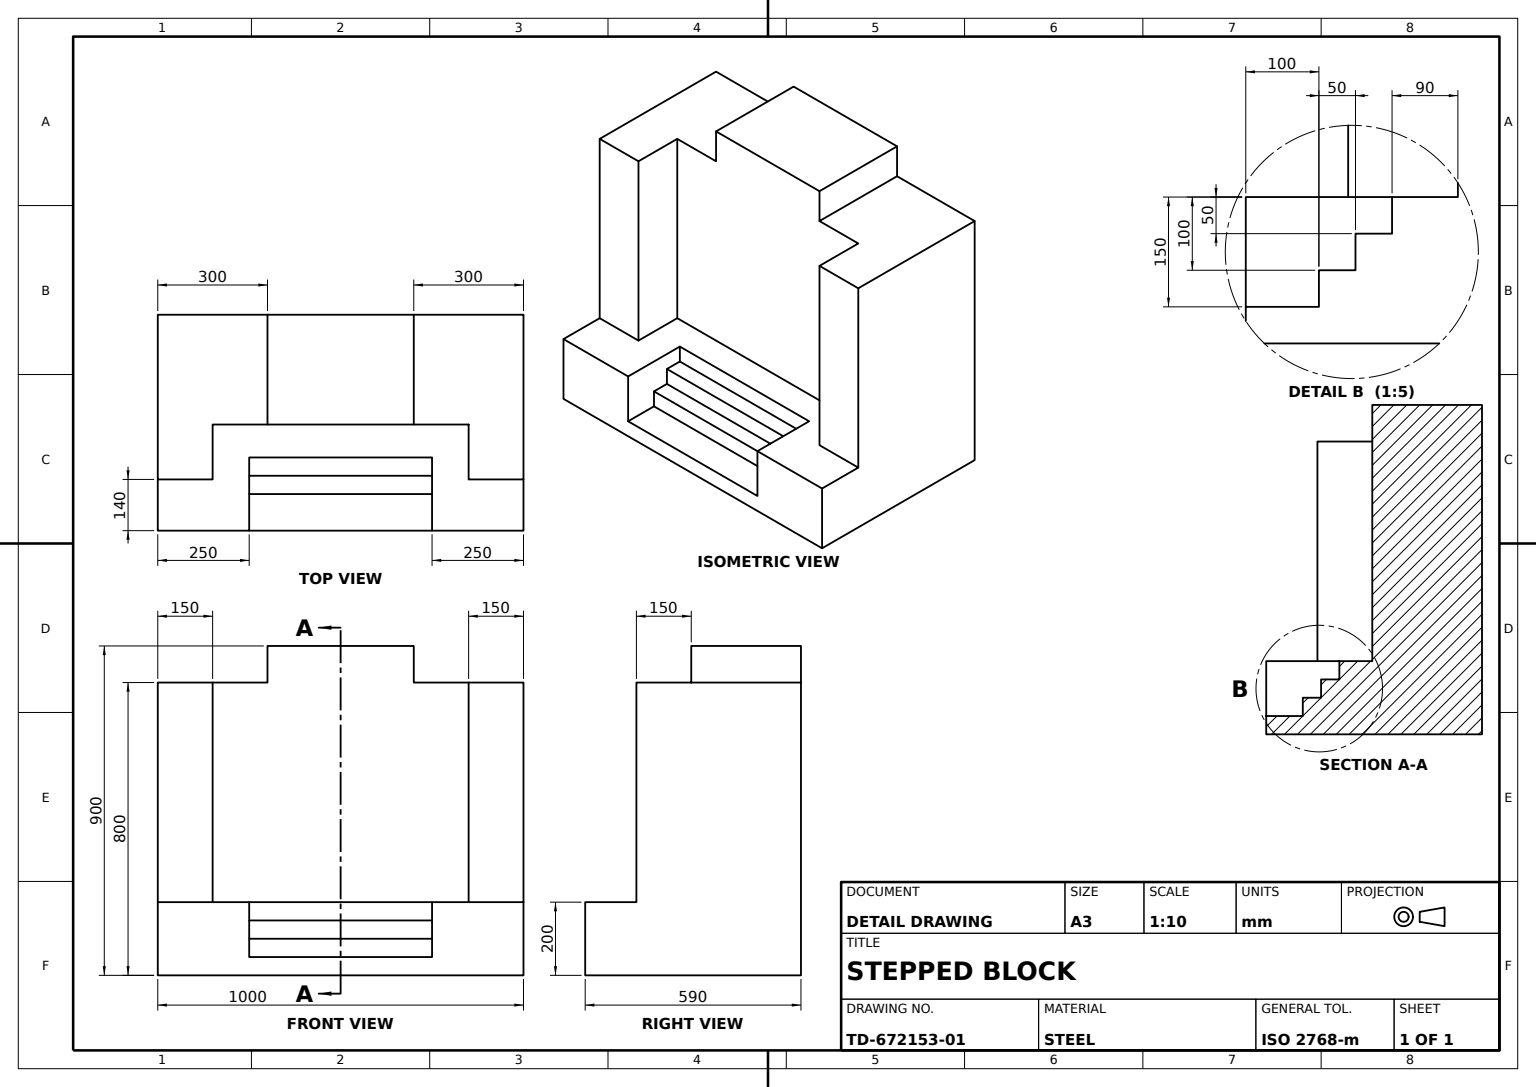
from build123d import *

# Parameters (mm, degrees)
BASE_BLOCK_DEPTH          = 1000
SIDE_BOSS_A_SKETCH_W      = 150
SIDE_BOSS_A_SKETCH_H      = 600
SIDE_BOSS_A_DEPTH         = 150
SIDE_BOSS_B_SKETCH_W      = 150
SIDE_BOSS_B_SKETCH_H      = 600
SIDE_BOSS_B_DEPTH         = 150
CORNER_BOSS_DEPTH         = 100
TOP_STEP_CUT_DEPTH        = 150
TOP_GROOVE_CUT_DEPTH      = 1450.689621954
TOP_GROOVE_CUT_DEPTH_BACK = 100
GROOVE_NOTCH_SKETCH_W     = 500
GROOVE_NOTCH_SKETCH_H     = 50
GROOVE_NOTCH_CUT_DEPTH    = 50
GROOVE_INFILL_BOSS_DEPTH  = 50


with BuildPart() as part:
    # Base Profile Sketch → Base Block (new body)
    with BuildSketch(Plane.XY):
        Polygon((0, 0), (540, 0), (540, 800), (240, 800), (240, 200), (0, 200), align=None)
    extrude(amount=BASE_BLOCK_DEPTH)

    # Side Boss A Sketch → Side Boss A (add)
    with BuildSketch(Plane(origin=(0, 0, 0), x_dir=(-1, 0, 0), z_dir=(0, 0, -1))):
        with Locations((-165, 500)):
            Rectangle(SIDE_BOSS_A_SKETCH_W, SIDE_BOSS_A_SKETCH_H)
    extrude(amount=-SIDE_BOSS_A_DEPTH)

    # Side Boss B Sketch → Side Boss B (add)
    with BuildSketch(Plane.XY.offset(1000)):
        with Locations((165, 500)):
            Rectangle(SIDE_BOSS_B_SKETCH_W, SIDE_BOSS_B_SKETCH_H)
    extrude(amount=-SIDE_BOSS_B_DEPTH)

    # Corner Boss Sketch → Corner Boss (add)
    with BuildSketch(Plane(origin=(0, 800, 0), x_dir=(1, 0, 0), z_dir=(0, 1, 0))):
        Polygon((540, -500), (540, -300), (240, -300), (240, -700), (540, -700), align=None)
    extrude(amount=CORNER_BOSS_DEPTH)

    # Top Step Cut Sketch → Top Step Cut (cut)
    with BuildSketch(Plane.ZY):
        Polygon((500, 200), (250, 200), (250, 150), (750, 150), (750, 200), align=None)
    extrude(amount=-TOP_STEP_CUT_DEPTH, mode=Mode.SUBTRACT)

    # Top Groove Sketch → Top Groove Cut (cut, two sides: drawn at the far end of the back side and taken through both)
    with BuildSketch(Plane.ZY.offset(-TOP_GROOVE_CUT_DEPTH_BACK)):
        Polygon((250, 2281.32034356), (250, 150), (250, 100), (750, 100), (750, 150), (750, 2281.32034356), (750, 6543.961030679), (250, 6543.961030679), align=None)
    extrude(amount=TOP_GROOVE_CUT_DEPTH + TOP_GROOVE_CUT_DEPTH_BACK, mode=Mode.SUBTRACT)

    # Groove Notch Sketch → Groove Notch Cut (cut)
    with BuildSketch(Plane.ZY):
        with Locations((500, 75)):
            Rectangle(GROOVE_NOTCH_SKETCH_W, GROOVE_NOTCH_SKETCH_H)
    extrude(amount=-GROOVE_NOTCH_CUT_DEPTH, mode=Mode.SUBTRACT)

    # Groove Infill Sketch → Groove Infill Boss (add)
    with BuildSketch(Plane.ZY):
        Polygon((0, 200), (0, 0), (1000, 0), (1000, 200), (750, 200), (750, 50), (250, 50), (250, 200), align=None)
    extrude(amount=GROOVE_INFILL_BOSS_DEPTH)


solid = part.part
